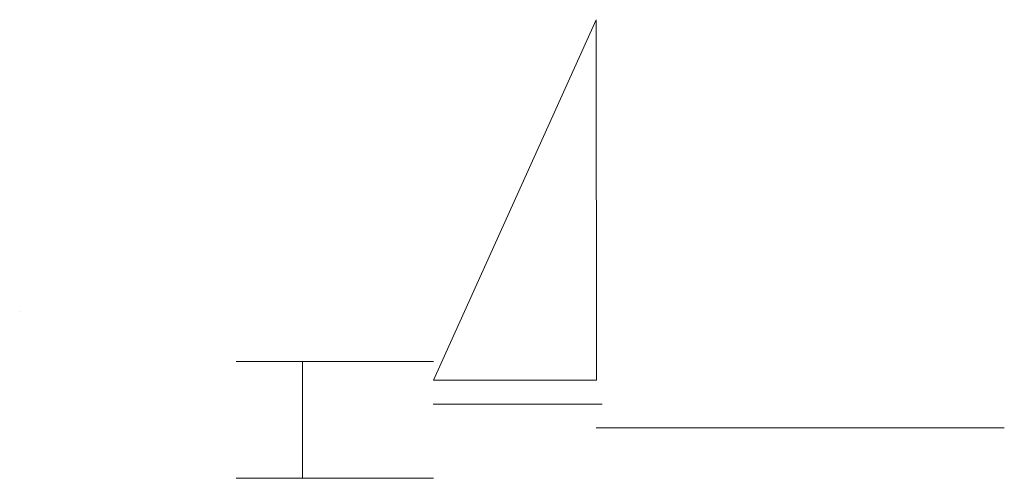
# Model space of a CAD drawing. Units: millimetres. Extents: x 103 to 289, y -10 to 77.
import ezdxf

# ---------------------------------------------------------------- set-up
doc = ezdxf.new("R2010")
doc.units = ezdxf.units.MM
doc.layers.add('M-CONS', color=8, linetype='Continuous', lineweight=13)

msp = doc.modelspace()

# ---------------------------------------------------------------- linework, layer by layer
at = {"layer": 'M-CONS', "extrusion": (0, -1, 0)}
for p, q in [((103.23, 22, 76.89), (103.23, 22, 76.89)), ((156.54, -9.5, 65.7), (156.54, 12.5, 65.7)), ((162.26, 12.5, 76.82), (181.26, 12.5, 76.82)), ((181.26, 12.5, 76.82), (181.26, 12.5, 54.82)), ((279.43, 0, 65.25), (241.63, 0, 51.16)), ((279.38, 0, 78.29), (241.64, 0, 92.39)), ((279.38, 0, 78.29), (279.38, 0, 78.29)), ((162.26, -9.5, 76.82), (162.26, -9.5, 76.82)), ((162.26, -9.5, 76.82), (181.26, -9.5, 76.82)), ((181.26, -9.5, 54.82), (162.68, -9.5, 54.82)), ((181.26, -9.5, 76.82), (181.26, -9.5, 54.82))]:
    msp.add_line(p, q, dxfattribs=at)
at = {"layer": 'M-CONS'}
msp.add_polyline3d([(212, 9, 70.82), (211.97, 77, 70.81), (181.26, 9, 70.82)], close=True, dxfattribs=at)
at = {"layer": 'M-CONS', "extrusion": (0, -1, 0)}
for centre, radius in [((156.54, 65.7, -12.5), 12.5), ((156.54, 65.7, -12.5), 6), ((233.95, 71.78), 22), ((233.95, 71.78), 18), ((281.95, 71.78), 7), ((281.95, 71.78), 5.5), ((156.54, 65.7, 9.5), 12.5), ((156.54, 65.7, 9.5), 6)]:
    msp.add_circle(centre, radius, dxfattribs=at)
msp.add_arc((233.95, 71.78), 22, 290.4354, 69.519, dxfattribs=at)
at = {"layer": 'M-CONS', "extrusion": (0, 1, 0)}
msp.add_rational_spline([(181.26, 4.5, 70.82), (181.26, 4.5, 73.82), (181.26, 4.5, 76.82), (196.89, 4.5, 76.82), (212.53, 4.5, 76.82), (212.53, 4.5, 73.76), (213.36, 4.5, 70.82), (197.31, 4.5, 70.82), (181.26, 4.5, 70.82)], [1, 1, 1, 1, 1, 0.990477507529, 1, 1, 1], degree=2, knots=[0, 0, 0, 1, 1, 2, 2, 2.276227, 2.276227, 3.276227, 3.276227, 3.276227], dxfattribs=at)

doc.saveas('drawing.dxf')
